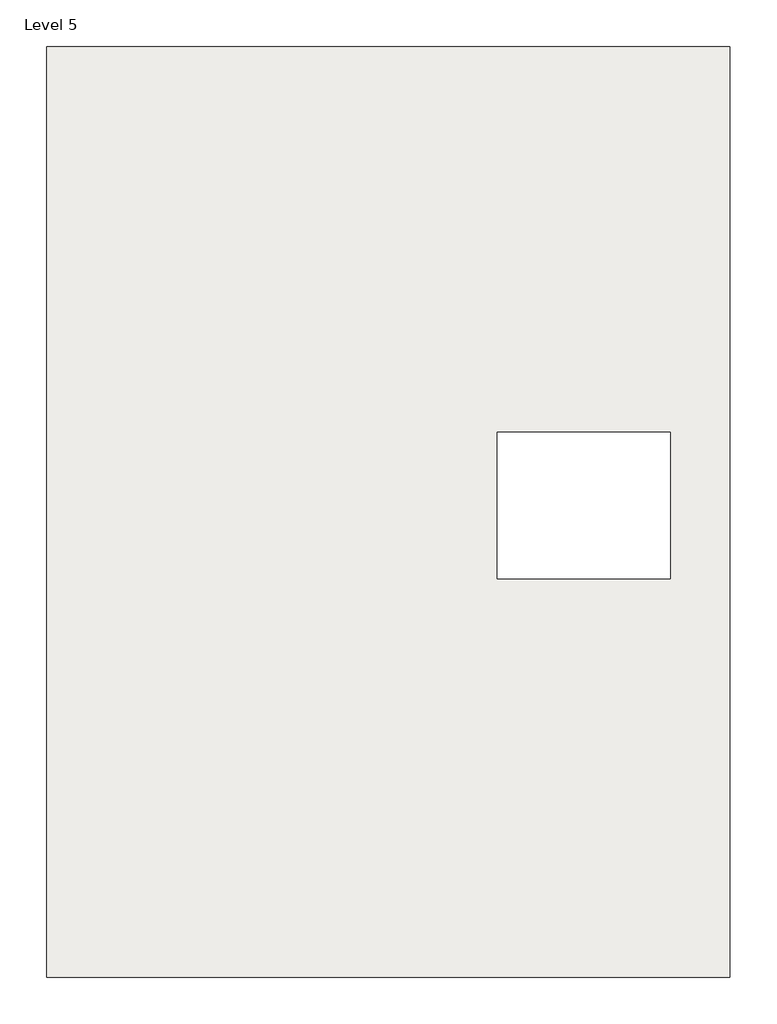
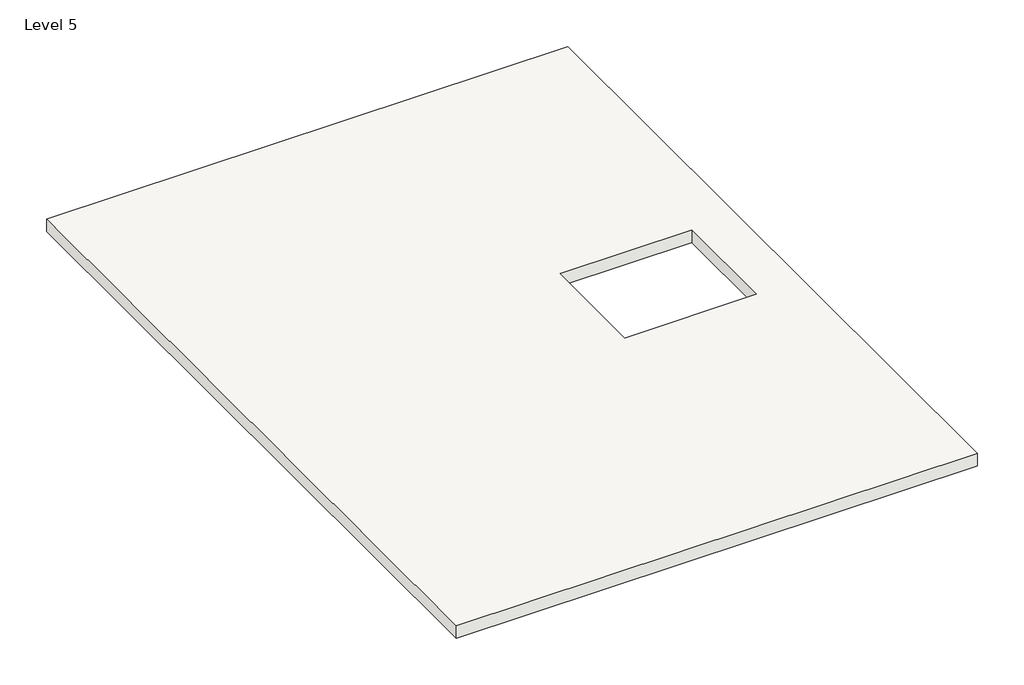
# One storey, incomplete: 1 roof.
"""IFC4 building model written with IfcOpenShell, lengths in millimetres."""

from ifc_helpers import new_model, si_unit, frame, origin, place, context, project, spatial, polyline, outline, extrude, element, save

model = new_model("IFC4")

# Units and contexts
model_context = context("Model", 3, world=origin())
ifc_project = project(units=[si_unit("LENGTHUNIT", "METRE", prefix="MILLI")], contexts=[model_context])

# Site, building, storey
site = spatial("IfcSite", under=ifc_project)
building = spatial("IfcBuilding", under=site)
storey = spatial("IfcBuildingStorey", under=building, Name="Level 5", Elevation=12192.0)

# Roof
placement = place(None, origin())
element("IfcRoof", 1, ObjectType="Generic - 12\"", at=placement, inside=storey, context=model_context, shape_type="SweptSolid", body=[
    extrude(outline(polyline([(-10475.6876145, -9022.8595056), (-10475.6876145, 7410.9404944), (1589.3123855, 7410.9404944), (1589.3123855, -9022.8595056), (-10475.6876145, -9022.8595056)]), holes=[polyline([(533.1774067, 602.8848622), (-2514.8225933, 602.8848622), (-2514.8225933, -1987.9151378), (533.1774067, -1987.9151378), (533.1774067, 602.8848622)])]), frame((0.0, 0.0, 12192.0), z_axis=(0.0, 0.0, 1.0), x_axis=(1.0, 0.0, 0.0)), (0.0, 0.0, 1.0), 304.8),
])

save(model, "model.ifc")

# Revit data of these elements
# Type "Generic - 12\""
#   Assembly Code = "B1020"
#   Layers, outside or top first: 1' - 0" no material (function 1)
# Element 1 (IfcRoof, "Generic - 12\"")
#   built-in parameter 1001705 = 41 (stored number, unit not read)
#   built-in parameter 1001710 = 33615
#   Phase Created = New Construction
#   Materials on its faces: "Default Roof"
# Materials
#   "Default Roof": colour RGB 88 101 114, transparency 0, Cost = 0
